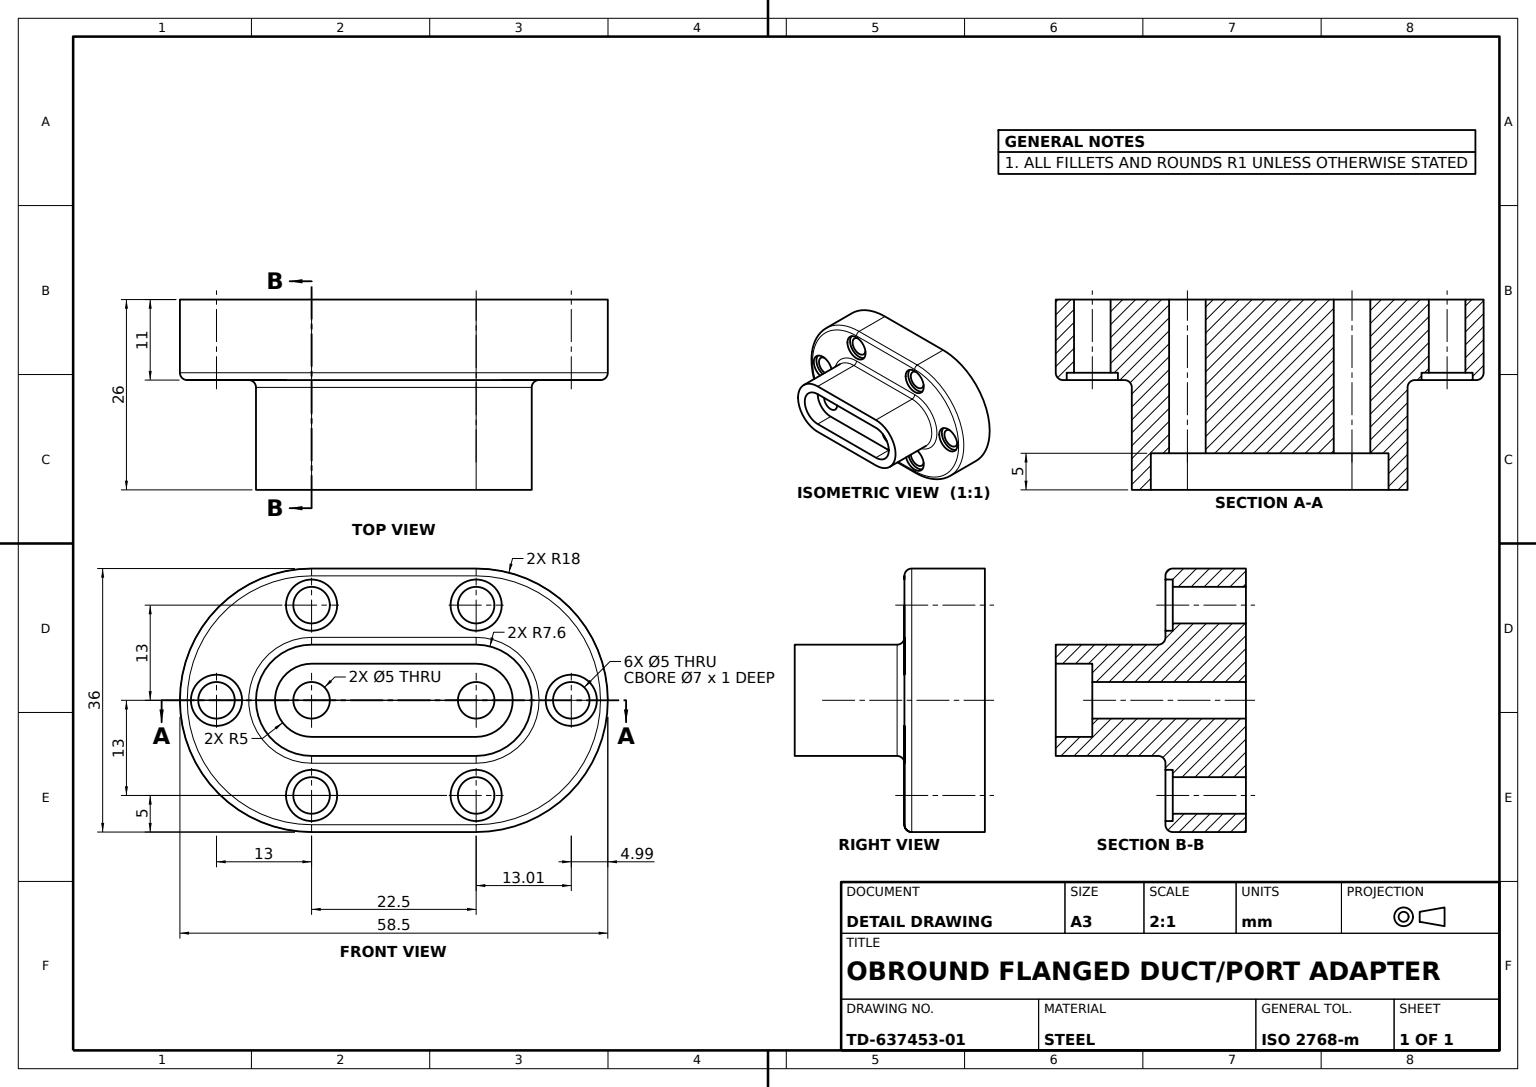
SolidWorks part; units mm, degrees
material "Plain Carbon Steel"
ref_plane "Front Plane" through (0, 0, 0) normal (0, 0, 1) x (1, 0, 0)
ref_plane "Top Plane" through (0, 0, 0) normal (0, 1, 0) x (1, 0, 0)
ref_plane "Right Plane" through (0, 0, 0) normal (1, 0, 0) x (0, 0, -1)
sketch "Flange Profile" plane through (0, 0, 0) normal (0, 0, 1) x (1, 0, 0)
  line L0 (0, 0) -> (22.5, 0) construction
  line L1 (0, 0) -> (22.5, 0) construction
  line L2 (0, 18) -> (22.5, 18)
  line L3 (0, -18) -> (22.5, -18)
  arc A0 (0, 18) -> (0, -18) centre (0, 0) ccw
  arc A1 (22.5, -18) -> (22.5, 18) centre (22.5, 0) ccw
  point P3 (11.25, 0)
  dimension "D2" = 18
  dimension "D1" = 22.5
extrude "Base Flange" add sketch "Flange Profile" along normal blind 11
sketch "Boss Profile" plane through (0, 0, 11) normal (0, 0, 1) x (1, 0, 0)
  line L0 (0, 0) -> (22.5, 0) construction
  line L1 (0, 7.6) -> (22.5, 7.6)
  line L2 (0, -7.6) -> (22.5, -7.6)
  line L3 (0, 0) -> (22.5, 0) construction
  arc A0 (0, 7.6) -> (0, -7.6) centre (0, 0) ccw
  arc A1 (22.5, -7.6) -> (22.5, 7.6) centre (22.5, 0) ccw
  point P4 (11.25, 0)
  point P11 (11.25, 0)
  dimension "D1" = 7.6
extrude "Obround Boss" add sketch "Boss Profile" along normal blind 15
sketch "Boss Pocket Profile" plane through (0, 0, 26) normal (0, 0, 1) x (1, 0, 0)
  line L0 (0, 0) -> (22.5, 0) construction
  line L1 (0, 5) -> (22.5, 5)
  line L2 (0, -5) -> (22.5, -5)
  arc A0 (0, 5) -> (0, -5) centre (0, 0) ccw
  arc A1 (22.5, -5) -> (22.5, 5) centre (22.5, 0) ccw
  point P4 (11.25, 0)
  dimension "D1" = 5
extrude "Boss Pocket" cut sketch "Boss Pocket Profile" against normal blind 5
sketch "Mounting Holes A Profile" plane through (0, 0, 11) normal (0, 0, 1) x (1, 0, 0)
  line L0 (0, 0) -> (22.5, 0) construction
  line L1 (0, 13) -> (22.5, 13) construction
  line L2 (0, -13) -> (22.5, -13) construction
  line L3 (0, -13) -> (0, 13) construction
  line L4 (22.5, 13) -> (22.5, -13) construction
  arc A0 (0, 13) -> (0, -13) centre (0, 0) ccw construction
  arc A1 (22.5, -13) -> (22.5, 13) centre (22.5, 0) ccw construction
  circle A2 centre (0, 13) radius 2.5
  circle A3 centre (22.5, 13) radius 2.5
  circle A4 centre (0, -13) radius 2.5
  circle A5 centre (22.5, -13) radius 2.5
  point P4 (11.25, 0)
  dimension "D1" = 13
  dimension "D2" = 5
  dimension "D3" = 5
  dimension "D4" = 5
  dimension "D5" = 5
extrude "Mounting Holes A" cut sketch "Mounting Holes A Profile" against normal through all
sketch "Spot Faces A Profile" plane through (0, 0, 11) normal (0, 0, 1) x (1, 0, 0)
  circle A0 centre (0, 13) radius 3.5
  circle A1 centre (22.5, 13) radius 3.5
  circle A2 centre (22.5, -13) radius 3.5
  circle A3 centre (0, -13) radius 3.5
  dimension "D1" = 7
  dimension "D2" = 7
  dimension "D3" = 7
  dimension "D4" = 7
extrude "Spot Faces A" cut sketch "Spot Faces A Profile" against normal blind 1
sketch "Centre Holes Profile" plane through (0, 0, 21) normal (0, 0, 1) x (1, 0, 0)
  circle A0 centre (0, 0) radius 2.5
  circle A1 centre (22.508, 0) radius 2.5
  arc A2 (22.5, -18) -> (22.5, 18) centre (22.5, 0) ccw construction
  dimension "D1" = 5
  dimension "D2" = 5
  dimension "D3" = 22.508
  dimension "D4" = 0.008
extrude "Centre Holes" cut sketch "Centre Holes Profile" against normal through all
fillet "Boss Root Fillet R1" radius 1 8 edges at (-18, 0, 11) (11.25, 18, 11) (40.5, 0, 11) (-7.6, 0, 11) (11.25, 7.6, 11) (30.1, 0, 11) (11.25, -18, 11) (11.25, -7.6, 11)
sketch "Mounting Holes B Profile" plane through (0, 0, 11) normal (0, 0, 1) x (1, 0, 0)
  line L0 (0, 0) -> (22.508, 0) construction
  line L1 (0, 13) -> (22.508, 13) construction
  line L2 (0, -13) -> (22.508, -13) construction
  line L3 (0, 0) -> (-13, 0) construction
  line L4 (22.508, 0) -> (35.508, 0) construction
  arc A0 (0, 13) -> (0, -13) centre (0, 0) ccw construction
  arc A1 (22.508, -13) -> (22.508, 13) centre (22.508, 0) ccw construction
  circle A2 centre (-13, 0) radius 2.5
  circle A3 centre (35.508, 0) radius 2.5
  point P4 (11.254, 0)
  dimension "D1" = 13
  dimension "D2" = 5
  dimension "D3" = 5
extrude "Mounting Holes B" cut sketch "Mounting Holes B Profile" against normal through all
sketch "Spot Faces B Profile" plane through (0, 0, 11) normal (0, 0, 1) x (1, 0, 0)
  circle A0 centre (-13, 0) radius 3.5
  circle A1 centre (35.508, 0) radius 3.5
  dimension "D1" = 7
  dimension "D2" = 7
extrude "Spot Faces B" cut sketch "Spot Faces B Profile" against normal blind 1
